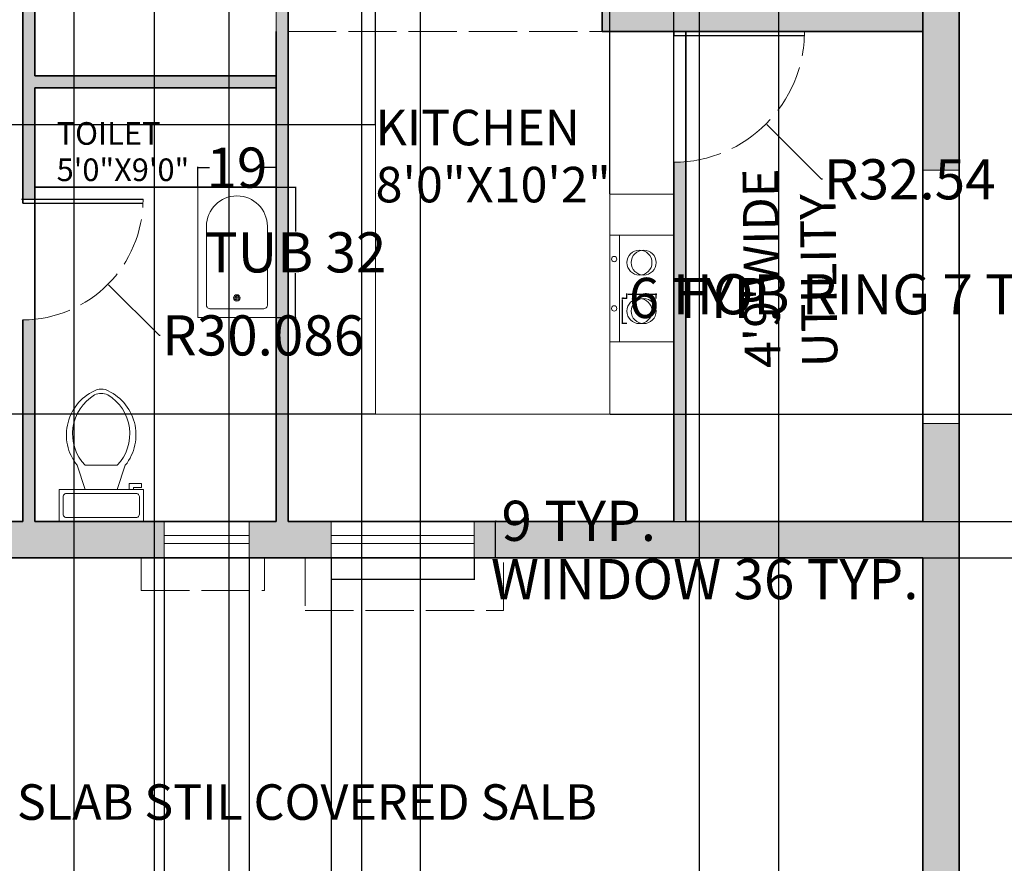
# Model space of a CAD drawing. Units: inches. Extents: x 300 to 1007, y 2 to 1069.
# Tile 9 of 12: x 617 to 862, y 533 to 743. Entities that reach past the tile are written whole.
import ezdxf

# ---------------------------------------------------------------- set-up
doc = ezdxf.new("R2010")
doc.units = ezdxf.units.IN
doc.header["$MEASUREMENT"] = 0
doc.linetypes.add('ACAD_ISO02W100', pattern=[15, 12, -3])
for name, color, linetype, lineweight in [('A-ANNO-DIMS', 2, 'Continuous', 18), ('A-ANNO-TEXT', 7, 'Continuous', 18), ('A-AREA-IDEN', 7, 'Continuous', 18), ('A-CASE', 8, 'Continuous', 18), ('A-DOOR', 3, 'Continuous', 25), ('A-DOOR-SWNG', 3, 'ACAD_ISO02W100', 13), ('A-EQPM', 9, 'Continuous', 18), ('A-FLOR-FIXT', 9, 'Continuous', 18), ('A-FLOR-SLAB', 7, 'Continuous', 35), ('A-GLAZ', 4, 'Continuous', 18), ('A-GLAZ-OVHD', 8, 'ACAD_ISO02W100', 13), ('A-WALL', 7, 'Continuous', 35), ('A-WALL-OVHD', 8, 'ACAD_ISO02W100', 18)]:
    doc.layers.add(name, color=color, linetype=linetype, lineweight=lineweight)
doc.layers.add('A-WALL-PATT', color=9, linetype='Continuous', lineweight=9, true_color=0xc7c8ca)
doc.styles.get("Standard").update_dxf_attribs({"font": 'arial.ttf'})
doc.dimstyles.get("Standard").update_dxf_attribs({"dimtxt": 10, "dimasz": 0.18, "dimexe": 0.18, "dimexo": 0.0625, "dimgap": 0.09, "dimtad": 0, "dimtih": 1, "dimtoh": 1, "dimdec": 0, "dimzin": 0, "dimdsep": 46, "dimlunit": 3, "dimtxsty": 'Standard', "dimcen": 0.09, "dimadec": 0, "dimazin": 0, "dimtfac": 1, "dimtdec": 0, "dimtofl": 0, "dimtmove": 0, "dimatfit": 3, "dimfxl": 1, "dimtolj": 1, "dimtzin": 0, "dimarcsym": 0})

# ---------------------------------------------------------------- blocks, each defined once
blk = doc.blocks.new('Bath Tub - 26 x 60 in.')
for p, q in [((8, -18), (10, -18)), ((9, -17), (9, -19))]:
    blk.add_line(p, q)
blk.add_lwpolyline([(0, -36), (0, 0), (60, 0), (60, -36)], close=True)
for points in [[(6, -4), (42, -4)], [(4, -30), (4, -6)], [(42, -32), (6, -32)]]:
    blk.add_lwpolyline(points)
for radius in [1.5, 1]:
    blk.add_circle((9, -18), radius)
for centre, radius, start, end in [((5.75, -5.75), 1.77, 81.8699, 188.1301), ((42, -18), 14, 270, 90), ((5.75, -30.25), 1.77, 171.8699, 278.1301)]:
    blk.add_arc(centre, radius, start, end)
blk = doc.blocks.new('Toilet - top')
for p, q in [((9.5, -6), (9.5, -2)), ((-10, -8.5), (-8, -8.5)), ((-10, -9.5), (-10, -8.5)), ((-7, -9.5), (-10, -9.5)), ((-8, -8.5), (-8, -8)), ((-7, -8), (-7, -9.5)), ((-4, -8), (-6, -14)), ((4, -8), (6, -14)), ((4, -14), (-4, -14))]:
    blk.add_line(p, q)
blk.add_lwpolyline([(10.5, -8), (10.5, 0), (-10.5, 0), (-10.5, -8)], close=True)
for points in [[(-9.5, -2), (-9.5, -6)], [(8.5, -1), (-8.5, -1)], [(-8.5, -7), (8.5, -7)]]:
    blk.add_lwpolyline(points)
for centre, radius, start, end in [((-8.62, -1.88), 0.884, 81.8699, 188.1301), ((8.62, -1.88), 0.884, 351.8699, 98.1301), ((-8.62, -6.12), 0.884, 171.8699, 278.1301), ((8.62, -6.12), 0.884, 261.8699, 8.1301), ((3.52, -21.58), 12.17, 141.4691, 247.9714), ((4.2, -21.82), 11.33, 136.3677, 238.9468), ((-3.52, -21.58), 12.17, 292.0284, 38.5307), ((-4.2, -21.82), 11.33, 301.053, 43.6321), ((0, -27.88), 4, 245.7318, 294.2682), ((0, -29), 4, 254.8605, 285.1395)]:
    blk.add_arc(centre, radius, start, end)
blk = doc.blocks.new('WIN-35_1-2')
for p, q in [((0, -4.5), (0, 4.5)), ((35.5, 0), (35.5, 4.5)), ((35.5, 4.5), (35.5, -4.5)), ((0, 1), (35.5, 1)), ((0, -1), (35.5, -1))]:
    blk.add_line(p, q)
blk = doc.blocks.new('COOKTOP-RING-6')
for centre in [(0, 0), (1.04, 0)]:
    blk.add_circle(centre, 3.11)
blk = doc.blocks.new('*D41')
at = {"layer": 'A-ANNO-DIMS', "color": 0, "lineweight": -2, "transparency": 16777216}
for p, q in [((680.89, 701.7), (685.87, 701.7)), ((685.69, 701.52), (685.69, 690.67)), ((685.69, 669.43), (685.69, 680.27)), ((680.89, 669.25), (685.87, 669.25))]:
    blk.add_line(p, q, dxfattribs=at)
at = {"layer": 'A-ANNO-DIMS', "color": 0, "transparency": 16777216}
for points in [[(685.66, 701.52), (685.72, 701.52), (685.69, 701.7)], [(685.66, 669.43), (685.72, 669.43), (685.69, 669.25)]]:
    blk.add_solid(points, dxfattribs=at)
at = {"layer": 'Defpoints', "color": 0, "transparency": 16777216}
for p in [(680.83, 701.7), (685.69, 701.7), (680.83, 669.25)]:
    blk.add_point(p, dxfattribs=at)
at = {"layer": 'A-ANNO-DIMS', "color": 0, "transparency": 16777216, "insert": (685.69, 685.47), "char_height": 10, "attachment_point": 5}
blk.add_mtext('\\A1;TUB 32', dxfattribs=at)
blk = doc.blocks.new('*D42')
at = {"layer": 'A-ANNO-DIMS', "color": 0, "lineweight": -2, "transparency": 16777216}
for p, q in [((661.36, 701.76), (661.36, 706.74)), ((661.54, 706.56), (664.3, 706.56)), ((680.65, 706.56), (677.88, 706.56)), ((680.83, 701.76), (680.83, 706.74))]:
    blk.add_line(p, q, dxfattribs=at)
at = {"layer": 'A-ANNO-DIMS', "color": 0, "transparency": 16777216}
for points in [[(661.54, 706.59), (661.54, 706.53), (661.36, 706.56)], [(680.65, 706.59), (680.65, 706.53), (680.83, 706.56)]]:
    blk.add_solid(points, dxfattribs=at)
at = {"layer": 'Defpoints', "color": 0, "transparency": 16777216}
for p in [(661.36, 706.56), (661.36, 701.7), (680.83, 701.7)]:
    blk.add_point(p, dxfattribs=at)
at = {"layer": 'A-ANNO-DIMS', "color": 0, "transparency": 16777216, "insert": (671.09, 706.56), "char_height": 10, "attachment_point": 5}
blk.add_mtext('\\A1;19', dxfattribs=at)
blk = doc.blocks.new('*D61')
at = {"layer": 'A-ANNO-DIMS', "color": 0, "lineweight": -2, "transparency": 16777216}
for p, q in [((694.58, 609.38), (694.58, 603.94)), ((730.11, 609.38), (730.11, 603.94)), ((694.76, 604.12), (729.93, 604.12)), ((730.11, 604.12), (730.29, 604.12))]:
    blk.add_line(p, q, dxfattribs=at)
at = {"layer": 'A-ANNO-DIMS', "color": 0, "transparency": 16777216}
for points in [[(694.76, 604.15), (694.76, 604.09), (694.58, 604.12)], [(729.93, 604.15), (729.93, 604.09), (730.11, 604.12)]]:
    blk.add_solid(points, dxfattribs=at)
at = {"layer": 'Defpoints', "color": 0, "transparency": 16777216}
for p in [(694.58, 609.45), (730.11, 609.45), (730.11, 604.12)]:
    blk.add_point(p, dxfattribs=at)
at = {"layer": 'A-ANNO-DIMS', "color": 0, "transparency": 16777216, "insert": (787.51, 604.12), "char_height": 10, "attachment_point": 5}
blk.add_mtext('\\A1;WINDOW 36 TYP.', dxfattribs=at)
blk = doc.blocks.new('*D62')
at = {"layer": 'A-ANNO-DIMS', "color": 0, "lineweight": -2, "transparency": 16777216}
for p, q in [((730.17, 618.45), (735.62, 618.45)), ((735.44, 618.45), (735.44, 618.63)), ((735.44, 618.63), (735.62, 618.63)), ((735.44, 609.63), (735.44, 618.27)), ((730.17, 609.45), (735.62, 609.45))]:
    blk.add_line(p, q, dxfattribs=at)
at = {"layer": 'A-ANNO-DIMS', "color": 0, "transparency": 16777216}
for points in [[(735.41, 618.27), (735.47, 618.27), (735.44, 618.45)], [(735.41, 609.63), (735.47, 609.63), (735.44, 609.45)]]:
    blk.add_solid(points, dxfattribs=at)
at = {"layer": 'Defpoints', "color": 0, "transparency": 16777216}
for p in [(730.11, 618.45), (735.44, 618.45), (730.11, 609.45)]:
    blk.add_point(p, dxfattribs=at)
at = {"layer": 'A-ANNO-DIMS', "color": 0, "transparency": 16777216, "insert": (756.16, 618.63), "char_height": 10, "attachment_point": 5}
blk.add_mtext('\\A1;9 TYP.', dxfattribs=at)
blk = doc.blocks.new('*D71')
at = {"layer": 'A-ANNO-DIMS', "color": 0, "lineweight": -2, "transparency": 16777216}
for p, q in [((768.17, 674), (768.17, 675.21)), ((768.35, 675.03), (775.25, 675.03)), ((775.43, 674), (775.43, 675.21)), ((775.43, 675.03), (775.61, 675.03))]:
    blk.add_line(p, q, dxfattribs=at)
at = {"layer": 'A-ANNO-DIMS', "color": 0, "transparency": 16777216}
for points in [[(768.35, 675.06), (768.35, 675), (768.17, 675.03)], [(775.25, 675.06), (775.25, 675), (775.43, 675.03)]]:
    blk.add_solid(points, dxfattribs=at)
at = {"layer": 'Defpoints', "color": 0, "transparency": 16777216}
for p in [(768.17, 673.94), (775.43, 675.03), (775.43, 673.94)]:
    blk.add_point(p, dxfattribs=at)
at = {"layer": 'A-ANNO-DIMS', "color": 0, "transparency": 16777216, "insert": (832.37, 675.03), "char_height": 10, "attachment_point": 5}
blk.add_mtext('\\A1;HOB RING 7 TYP.', dxfattribs=at)
blk = doc.blocks.new('*D72')
at = {"layer": 'A-ANNO-DIMS', "color": 0, "lineweight": -2, "transparency": 16777216}
for p, q in [((768.11, 673.94), (766.91, 673.94)), ((767.09, 673.94), (767.09, 674.12)), ((767.09, 674.12), (767.27, 674.12)), ((767.09, 667.9), (767.09, 673.76)), ((768.11, 667.72), (766.91, 667.72))]:
    blk.add_line(p, q, dxfattribs=at)
at = {"layer": 'A-ANNO-DIMS', "color": 0, "transparency": 16777216}
for points in [[(767.06, 673.76), (767.12, 673.76), (767.09, 673.94)], [(767.06, 667.9), (767.12, 667.9), (767.09, 667.72)]]:
    blk.add_solid(points, dxfattribs=at)
at = {"layer": 'Defpoints', "color": 0, "transparency": 16777216}
for p in [(767.09, 673.94), (768.17, 673.94), (768.17, 667.72)]:
    blk.add_point(p, dxfattribs=at)
at = {"layer": 'A-ANNO-DIMS', "color": 0, "transparency": 16777216, "insert": (787.84, 674.12), "char_height": 10, "attachment_point": 5}
blk.add_mtext('\\A1;6 TYP.', dxfattribs=at)
blk = doc.blocks.new('*D77')
at = {"layer": 'A-ANNO-DIMS', "color": 0, "lineweight": -2, "transparency": 16777216}
for p, q in [((841.89, 609.45), (974.48, 609.45)), ((974.3, 609.27), (974.3, 551.11)), ((974.3, 482.56), (974.3, 540.72)), ((850.89, 482.38), (974.48, 482.38))]:
    blk.add_line(p, q, dxfattribs=at)
at = {"layer": 'A-ANNO-DIMS', "color": 0, "transparency": 16777216}
for points in [[(974.27, 609.27), (974.33, 609.27), (974.3, 609.45)], [(974.27, 482.56), (974.33, 482.56), (974.3, 482.38)]]:
    blk.add_solid(points, dxfattribs=at)
at = {"layer": 'Defpoints', "color": 0, "transparency": 16777216}
for p in [(841.83, 609.45), (974.3, 609.45), (850.83, 482.38)]:
    blk.add_point(p, dxfattribs=at)
at = {"layer": 'A-ANNO-DIMS', "color": 0, "transparency": 16777216, "insert": (974.3, 545.92), "char_height": 10, "attachment_point": 5}
blk.add_mtext('\\A1;127.06', dxfattribs=at)
blk = doc.blocks.new('*D78')
at = {"layer": 'A-ANNO-DIMS', "color": 0, "lineweight": -2, "transparency": 16777216}
for p, q in [((850.89, 999.45), (974.48, 999.45)), ((974.3, 999.27), (974.3, 809.65)), ((974.3, 609.63), (974.3, 799.25)), ((841.89, 609.45), (974.48, 609.45))]:
    blk.add_line(p, q, dxfattribs=at)
at = {"layer": 'A-ANNO-DIMS', "color": 0, "transparency": 16777216}
for points in [[(974.27, 999.27), (974.33, 999.27), (974.3, 999.45)], [(974.27, 609.63), (974.33, 609.63), (974.3, 609.45)]]:
    blk.add_solid(points, dxfattribs=at)
at = {"layer": 'Defpoints', "color": 0, "transparency": 16777216}
for p in [(850.83, 999.45), (974.3, 999.45), (841.83, 609.45)]:
    blk.add_point(p, dxfattribs=at)
at = {"layer": 'A-ANNO-DIMS', "color": 0, "transparency": 16777216, "insert": (974.3, 804.45), "char_height": 10, "attachment_point": 5}
blk.add_mtext('\\A1;390', dxfattribs=at)
blk = doc.blocks.new('*D80')
at = {"layer": 'A-ANNO-DIMS', "color": 0, "lineweight": -2, "transparency": 16777216}
for p, q in [((683.83, 717.31), (683.83, 1063.03)), ((684.01, 1062.85), (705.41, 1062.85)), ((705.59, 717.31), (705.59, 1063.03)), ((705.59, 1062.85), (705.77, 1062.85))]:
    blk.add_line(p, q, dxfattribs=at)
at = {"layer": 'A-ANNO-DIMS', "color": 0, "transparency": 16777216}
for points in [[(684.01, 1062.88), (684.01, 1062.82), (683.83, 1062.85)], [(705.41, 1062.88), (705.41, 1062.82), (705.59, 1062.85)]]:
    blk.add_solid(points, dxfattribs=at)
at = {"layer": 'Defpoints', "color": 0, "transparency": 16777216}
for p in [(705.59, 1062.85), (683.83, 717.25), (705.59, 717.25)]:
    blk.add_point(p, dxfattribs=at)
at = {"layer": 'A-ANNO-DIMS', "color": 0, "transparency": 16777216, "insert": (726.71, 1062.85), "char_height": 10, "attachment_point": 5}
blk.add_mtext('\\A1;21.767', dxfattribs=at)
blk = doc.blocks.new('*D81')
at = {"layer": 'A-ANNO-DIMS', "color": 0, "lineweight": -2, "transparency": 16777216}
for p, q in [((705.53, 717.25), (354.19, 717.25)), ((354.37, 717.07), (354.37, 686.41)), ((354.37, 645.35), (354.37, 676.01)), ((705.53, 645.17), (354.19, 645.17))]:
    blk.add_line(p, q, dxfattribs=at)
at = {"layer": 'A-ANNO-DIMS', "color": 0, "transparency": 16777216}
for points in [[(354.34, 717.07), (354.4, 717.07), (354.37, 717.25)], [(354.34, 645.35), (354.4, 645.35), (354.37, 645.17)]]:
    blk.add_solid(points, dxfattribs=at)
at = {"layer": 'Defpoints', "color": 0, "transparency": 16777216}
for p in [(354.37, 717.25), (705.59, 717.25), (705.59, 645.17)]:
    blk.add_point(p, dxfattribs=at)
at = {"layer": 'A-ANNO-DIMS', "color": 0, "transparency": 16777216, "insert": (354.37, 681.21), "char_height": 10, "attachment_point": 5}
blk.add_mtext('\\A1;72.08', dxfattribs=at)
blk = doc.blocks.new('*D82')
at = {"layer": 'A-ANNO-DIMS', "color": 0, "lineweight": -2, "transparency": 16777216}
for p, q in [((763.9, 700.01), (763.9, 1063.03)), ((764.08, 1062.85), (779.65, 1062.85)), ((779.83, 700.01), (779.83, 1063.03)), ((779.83, 1062.85), (780.01, 1062.85))]:
    blk.add_line(p, q, dxfattribs=at)
at = {"layer": 'A-ANNO-DIMS', "color": 0, "transparency": 16777216}
for points in [[(764.08, 1062.88), (764.08, 1062.82), (763.9, 1062.85)], [(779.65, 1062.88), (779.65, 1062.82), (779.83, 1062.85)]]:
    blk.add_solid(points, dxfattribs=at)
at = {"layer": 'Defpoints', "color": 0, "transparency": 16777216}
for p in [(779.83, 1062.85), (763.9, 699.95), (779.83, 699.95)]:
    blk.add_point(p, dxfattribs=at)
at = {"layer": 'A-ANNO-DIMS', "color": 0, "transparency": 16777216, "insert": (800.38, 1062.85), "char_height": 10, "attachment_point": 5}
blk.add_mtext('\\A1;15.927', dxfattribs=at)
blk = doc.blocks.new('*D83')
at = {"layer": 'A-ANNO-DIMS', "color": 0, "lineweight": -2, "transparency": 16777216}
for p, q in [((763.96, 645.17), (974.48, 645.17)), ((974.3, 644.99), (974.3, 637)), ((974.3, 618.63), (974.3, 626.61)), ((779.89, 618.45), (974.48, 618.45))]:
    blk.add_line(p, q, dxfattribs=at)
at = {"layer": 'A-ANNO-DIMS', "color": 0, "transparency": 16777216}
for points in [[(974.27, 644.99), (974.33, 644.99), (974.3, 645.17)], [(974.27, 618.63), (974.33, 618.63), (974.3, 618.45)]]:
    blk.add_solid(points, dxfattribs=at)
at = {"layer": 'Defpoints', "color": 0, "transparency": 16777216}
for p in [(763.9, 645.17), (974.3, 645.17), (779.83, 618.45)]:
    blk.add_point(p, dxfattribs=at)
at = {"layer": 'A-ANNO-DIMS', "color": 0, "transparency": 16777216, "insert": (974.3, 631.81), "char_height": 10, "attachment_point": 5}
blk.add_mtext('\\A1;26.72', dxfattribs=at)
blk = doc.blocks.new('*D86')
at = {"layer": 'A-ANNO-DIMS', "color": 0, "lineweight": -2, "transparency": 16777216}
for p, q in [((805.95, 235.15), (805.95, 1063.03)), ((806.13, 1062.85), (822.02, 1062.85)), ((864.07, 1062.85), (848.18, 1062.85)), ((864.25, 235.15), (864.25, 1063.03))]:
    blk.add_line(p, q, dxfattribs=at)
at = {"layer": 'A-ANNO-DIMS', "color": 0, "transparency": 16777216}
for points in [[(806.13, 1062.88), (806.13, 1062.82), (805.95, 1062.85)], [(864.07, 1062.88), (864.07, 1062.82), (864.25, 1062.85)]]:
    blk.add_solid(points, dxfattribs=at)
at = {"layer": 'Defpoints', "color": 0, "transparency": 16777216}
for p in [(864.25, 1062.85), (805.95, 235.08), (864.25, 235.08)]:
    blk.add_point(p, dxfattribs=at)
at = {"layer": 'A-ANNO-DIMS', "color": 0, "transparency": 16777216, "insert": (835.1, 1062.85), "char_height": 10, "attachment_point": 5}
blk.add_mtext('\\A1;58.3', dxfattribs=at)
blk = doc.blocks.new('*D99')
at = {"layer": 'A-ANNO-DIMS', "color": 0, "lineweight": -2, "transparency": 16777216}
for p, q in [((604.49, 482.45), (604.49, 1063.03)), ((604.67, 1062.85), (619.83, 1062.85)), ((668.97, 1062.85), (653.8, 1062.85)), ((669.15, 482.45), (669.15, 1063.03))]:
    blk.add_line(p, q, dxfattribs=at)
at = {"layer": 'A-ANNO-DIMS', "color": 0, "transparency": 16777216}
for points in [[(604.67, 1062.88), (604.67, 1062.82), (604.49, 1062.85)], [(668.97, 1062.88), (668.97, 1062.82), (669.15, 1062.85)]]:
    blk.add_solid(points, dxfattribs=at)
at = {"layer": 'Defpoints', "color": 0, "transparency": 16777216}
for p in [(669.15, 1062.85), (604.49, 482.38), (669.15, 482.38)]:
    blk.add_point(p, dxfattribs=at)
at = {"layer": 'A-ANNO-DIMS', "color": 0, "transparency": 16777216, "insert": (636.82, 1062.85), "char_height": 10, "attachment_point": 5}
blk.add_mtext('\\A1;64.66', dxfattribs=at)
blk = doc.blocks.new('*D100')
at = {"layer": 'A-ANNO-DIMS', "color": 0, "lineweight": -2, "transparency": 16777216}
for p, q in [((716.78, 482.45), (716.78, 1063.03)), ((716.96, 1062.85), (734.53, 1062.85)), ((786.04, 1062.85), (768.47, 1062.85)), ((786.22, 482.45), (786.22, 1063.03))]:
    blk.add_line(p, q, dxfattribs=at)
at = {"layer": 'A-ANNO-DIMS', "color": 0, "transparency": 16777216}
for points in [[(716.96, 1062.88), (716.96, 1062.82), (716.78, 1062.85)], [(786.04, 1062.88), (786.04, 1062.82), (786.22, 1062.85)]]:
    blk.add_solid(points, dxfattribs=at)
at = {"layer": 'Defpoints', "color": 0, "transparency": 16777216}
for p in [(786.22, 1062.85), (716.78, 482.38), (786.22, 482.38)]:
    blk.add_point(p, dxfattribs=at)
at = {"layer": 'A-ANNO-DIMS', "color": 0, "transparency": 16777216, "insert": (751.5, 1062.85), "char_height": 10, "attachment_point": 5}
blk.add_mtext('\\A1;69.44', dxfattribs=at)
blk = doc.blocks.new('*D102')
at = {"layer": 'A-ANNO-DIMS', "color": 0, "lineweight": -2, "transparency": 16777216}
for p, q in [((600.34, 609.38), (600.34, 8.45)), ((652.99, 609.38), (652.99, 8.45)), ((600.52, 8.63), (609.71, 8.63)), ((652.81, 8.63), (643.62, 8.63))]:
    blk.add_line(p, q, dxfattribs=at)
at = {"layer": 'A-ANNO-DIMS', "color": 0, "transparency": 16777216}
for points in [[(600.52, 8.66), (600.52, 8.6), (600.34, 8.63)], [(652.81, 8.66), (652.81, 8.6), (652.99, 8.63)]]:
    blk.add_solid(points, dxfattribs=at)
at = {"layer": 'Defpoints', "color": 0, "transparency": 16777216}
for p in [(600.34, 609.45), (652.99, 609.45), (652.99, 8.63)]:
    blk.add_point(p, dxfattribs=at)
at = {"layer": 'A-ANNO-DIMS', "color": 0, "transparency": 16777216, "insert": (626.66, 8.63), "char_height": 10, "attachment_point": 5}
blk.add_mtext('\\A1;52.66', dxfattribs=at)
blk = doc.blocks.new('*D103')
at = {"layer": 'A-ANNO-DIMS', "color": 0, "lineweight": -2, "transparency": 16777216}
for p, q in [((652.99, 609.38), (652.99, 8.45)), ((674.16, 609.38), (674.16, 8.45)), ((653.17, 8.63), (673.98, 8.63)), ((674.16, 8.63), (674.34, 8.63))]:
    blk.add_line(p, q, dxfattribs=at)
at = {"layer": 'A-ANNO-DIMS', "color": 0, "transparency": 16777216}
for points in [[(653.17, 8.66), (653.17, 8.6), (652.99, 8.63)], [(673.98, 8.66), (673.98, 8.6), (674.16, 8.63)]]:
    blk.add_solid(points, dxfattribs=at)
at = {"layer": 'Defpoints', "color": 0, "transparency": 16777216}
for p in [(652.99, 609.45), (674.16, 609.45), (674.16, 8.63)]:
    blk.add_point(p, dxfattribs=at)
at = {"layer": 'A-ANNO-DIMS', "color": 0, "transparency": 16777216, "insert": (695.25, 8.63), "char_height": 10, "attachment_point": 5}
blk.add_mtext('\\A1;21.164', dxfattribs=at)
blk = doc.blocks.new('*D104')
at = {"layer": 'A-ANNO-DIMS', "color": 0, "lineweight": -2, "transparency": 16777216}
for p, q in [((674.16, 609.38), (674.16, 8.45)), ((694.58, 609.38), (694.58, 8.45)), ((674.34, 8.63), (694.4, 8.63)), ((694.58, 8.63), (694.76, 8.63))]:
    blk.add_line(p, q, dxfattribs=at)
at = {"layer": 'A-ANNO-DIMS', "color": 0, "transparency": 16777216}
for points in [[(674.34, 8.66), (674.34, 8.6), (674.16, 8.63)], [(694.4, 8.66), (694.4, 8.6), (694.58, 8.63)]]:
    blk.add_solid(points, dxfattribs=at)
at = {"layer": 'Defpoints', "color": 0, "transparency": 16777216}
for p in [(674.16, 609.45), (694.58, 609.45), (694.58, 8.63)]:
    blk.add_point(p, dxfattribs=at)
at = {"layer": 'A-ANNO-DIMS', "color": 0, "transparency": 16777216, "insert": (711.75, 8.63), "char_height": 10, "attachment_point": 5}
blk.add_mtext('\\A1;20.42', dxfattribs=at)
blk = doc.blocks.new('*D106')
at = {"layer": 'A-ANNO-DIMS', "color": 0, "lineweight": -2, "transparency": 16777216}
for p, q in [((582.11, 990.38), (582.11, 8.45)), ((630.49, 990.38), (630.49, 8.45)), ((582.29, 8.63), (589.12, 8.63)), ((630.31, 8.63), (623.47, 8.63))]:
    blk.add_line(p, q, dxfattribs=at)
at = {"layer": 'A-ANNO-DIMS', "color": 0, "transparency": 16777216}
for points in [[(582.29, 8.66), (582.29, 8.6), (582.11, 8.63)], [(630.31, 8.66), (630.31, 8.6), (630.49, 8.63)]]:
    blk.add_solid(points, dxfattribs=at)
at = {"layer": 'Defpoints', "color": 0, "transparency": 16777216}
for p in [(582.11, 990.45), (630.49, 990.45), (630.49, 8.63)]:
    blk.add_point(p, dxfattribs=at)
at = {"layer": 'A-ANNO-DIMS', "color": 0, "transparency": 16777216, "insert": (606.3, 8.63), "char_height": 10, "attachment_point": 5}
blk.add_mtext('\\A1;48.38', dxfattribs=at)
blk = doc.blocks.new('*D107')
at = {"layer": 'A-ANNO-DIMS', "color": 0, "lineweight": -2, "transparency": 16777216}
for p, q in [((630.49, 990.38), (630.49, 8.45)), ((650.47, 990.38), (650.47, 8.45)), ((630.67, 8.63), (650.29, 8.63)), ((650.47, 8.63), (650.65, 8.63))]:
    blk.add_line(p, q, dxfattribs=at)
at = {"layer": 'A-ANNO-DIMS', "color": 0, "transparency": 16777216}
for points in [[(630.67, 8.66), (630.67, 8.6), (630.49, 8.63)], [(650.29, 8.66), (650.29, 8.6), (650.47, 8.63)]]:
    blk.add_solid(points, dxfattribs=at)
at = {"layer": 'Defpoints', "color": 0, "transparency": 16777216}
for p in [(630.49, 990.45), (650.47, 990.45), (650.47, 8.63)]:
    blk.add_point(p, dxfattribs=at)
at = {"layer": 'A-ANNO-DIMS', "color": 0, "transparency": 16777216, "insert": (667.15, 8.63), "char_height": 10, "attachment_point": 5}
blk.add_mtext('\\A1;19.98', dxfattribs=at)
blk = doc.blocks.new('*D108')
at = {"layer": 'A-ANNO-DIMS', "color": 0, "lineweight": -2, "transparency": 16777216}
for p, q in [((650.47, 990.38), (650.47, 8.45)), ((702.09, 990.38), (702.09, 8.45)), ((650.65, 8.63), (659.37, 8.63)), ((701.91, 8.63), (693.19, 8.63))]:
    blk.add_line(p, q, dxfattribs=at)
at = {"layer": 'A-ANNO-DIMS', "color": 0, "transparency": 16777216}
for points in [[(650.65, 8.66), (650.65, 8.6), (650.47, 8.63)], [(701.91, 8.66), (701.91, 8.6), (702.09, 8.63)]]:
    blk.add_solid(points, dxfattribs=at)
at = {"layer": 'Defpoints', "color": 0, "transparency": 16777216}
for p in [(650.47, 990.45), (702.09, 990.45), (702.09, 8.63)]:
    blk.add_point(p, dxfattribs=at)
at = {"layer": 'A-ANNO-DIMS', "color": 0, "transparency": 16777216, "insert": (676.28, 8.63), "char_height": 10, "attachment_point": 5}
blk.add_mtext('\\A1;51.62', dxfattribs=at)
blk = doc.blocks.new('*D115')
at = {"layer": 'A-ANNO-DIMS', "color": 0, "lineweight": -2, "transparency": 16777216}
for p, q in [((779.7, 740.45), (779.88, 740.45)), ((779.79, 740.36), (779.79, 740.54)), ((816.62, 703.66), (802.94, 717.33)), ((816.8, 703.66), (816.62, 703.66))]:
    blk.add_line(p, q, dxfattribs=at)
at = {"layer": 'A-ANNO-DIMS', "color": 0, "transparency": 16777216}
blk.add_solid([(802.96, 717.35), (802.92, 717.3), (802.81, 717.45)], dxfattribs=at)
at = {"layer": 'Defpoints', "color": 0, "transparency": 16777216}
for p in [(779.79, 740.45), (802.81, 717.45)]:
    blk.add_point(p, dxfattribs=at)
at = {"layer": 'A-ANNO-DIMS', "color": 0, "transparency": 16777216, "insert": (838.53, 703.66), "char_height": 10, "attachment_point": 5}
blk.add_mtext('\\A1;R32.54', dxfattribs=at)
blk = doc.blocks.new('*D117')
at = {"layer": 'A-ANNO-DIMS', "color": 0, "lineweight": -2, "transparency": 16777216}
for p, q in [((617.56, 698.73), (617.74, 698.73)), ((617.65, 698.64), (617.65, 698.82)), ((651.79, 664.79), (639.12, 677.39)), ((651.97, 664.79), (651.79, 664.79))]:
    blk.add_line(p, q, dxfattribs=at)
at = {"layer": 'A-ANNO-DIMS', "color": 0, "transparency": 16777216}
blk.add_solid([(639.14, 677.41), (639.09, 677.37), (638.99, 677.52)], dxfattribs=at)
at = {"layer": 'Defpoints', "color": 0, "transparency": 16777216}
for p in [(617.65, 698.73), (638.99, 677.52)]:
    blk.add_point(p, dxfattribs=at)
at = {"layer": 'A-ANNO-DIMS', "color": 0, "transparency": 16777216, "insert": (677.6, 664.79), "char_height": 10, "attachment_point": 5}
blk.add_mtext('\\A1;R30.086', dxfattribs=at)

msp = doc.modelspace()

# ---------------------------------------------------------------- hatches: boundary and pattern name
at = {"layer": 'A-WALL-PATT'}
h = msp.add_hatch(color=256, dxfattribs=at)
h.dxf.hatch_style = 1
h.paths.add_polyline_path([(546.104, 999.4468), (478.8267, 999.4468), (478.8267, 869.2798, -0.06322715), (487.8267, 868.1328), (487.8267, 990.4468), (546.104, 990.4468)])
h.paths.add_polyline_path([(630.4852, 999.4468), (582.106, 999.4468), (582.106, 990.4468), (613.8267, 990.4468), (613.8267, 867.4468), (622.8267, 867.4468), (622.8267, 990.4468), (630.4852, 990.4468)])
h.paths.add_polyline_path([(702.0883, 999.4468), (650.4653, 999.4468), (650.4653, 990.4468), (682.8267, 990.4468), (682.8267, 960.0824, -0.02530575), (685.8267, 960.0478), (685.8267, 990.4468), (702.0883, 990.4468)])
h.paths.add_polyline_path([(850.8267, 999.4468), (737.5888, 999.4468), (737.5888, 990.4468), (841.8267, 990.4468), (841.8267, 950.5685), (850.8267, 950.5685)])
h.paths.add_polyline_path([(685.8267, 930.4465), (682.8267, 930.4465), (682.8267, 888.4468), (682.8267, 867.4468), (685.8267, 867.4468), (697.4169, 867.4468), (697.4169, 870.4468), (685.8267, 870.4468), (685.8267, 888.4468)])
h.paths.add_polyline_path([(682.8267, 931.4465), (654.3436, 931.4465, 0.00843109), (654.3267, 930.4465), (682.8267, 930.4465)])
h.paths.add_polyline_path([(685.8267, 931.4465), (682.8267, 931.4465), (682.8267, 930.4465), (685.8267, 930.4465)])
h.paths.add_polyline_path([(682.8267, 888.4468), (622.8267, 888.4468), (622.8267, 885.4468), (682.8267, 885.4468)])
h.paths.add_polyline_path([(850.8267, 870.4468), (850.8267, 914.7851), (841.8267, 914.7851), (841.8267, 870.4468), (732.7101, 870.4468, -0.02120595), (732.8267, 867.4468), (779.8267, 867.4468), (779.8267, 749.4468), (782.8267, 749.4468), (788.8267, 749.4468), (788.8267, 861.4468), (841.8267, 861.4468), (841.8267, 749.4468), (850.8267, 749.4468)])
h.paths.add_polyline_path([(622.8267, 810.4468), (487.8267, 810.4468), (487.8267, 833.2626), (478.8267, 833.2626), (478.8267, 609.4468), (478.8267, 482.3847), (487.8267, 482.3847), (487.8267, 801.4468), (620.8267, 801.4468), (622.8267, 801.4468)])
h.paths.add_polyline_path([(680.8267, 729.4468), (620.8267, 729.4468), (620.8267, 765.8246, -0.02111352), (617.8267, 766.0562), (617.8267, 698.7303), (620.8267, 698.7303), (620.8267, 726.4468), (680.8267, 726.4468)])
h.paths.add_polyline_path([(620.8267, 668.8122, -0.02498293), (617.8267, 668.6448), (617.8267, 618.4468), (600.3357, 618.4468), (600.3357, 609.4468), (652.9929, 609.4468), (652.9929, 618.4468), (620.8267, 618.4468)])
h.paths.add_polyline_path([(552.3393, 618.4468), (487.8267, 618.4468), (487.8267, 609.4468), (552.3393, 609.4468)], flags=17)
h.paths.add_polyline_path([(694.5763, 618.4468), (683.8267, 618.4468), (683.8267, 726.4468), (683.8267, 749.4468), (680.8267, 749.4468), (680.8267, 740.4468), (680.8267, 726.4468), (680.8267, 618.4468), (674.1573, 618.4468), (674.1573, 609.4468), (680.8267, 609.4468), (694.5763, 609.4468)])
h.paths.add_polyline_path([(850.8267, 642.8902), (841.8267, 642.8902), (841.8267, 618.4468), (782.8267, 618.4468), (782.8267, 708.0513, -0.02308839), (779.8267, 707.9092), (779.8267, 618.4468), (730.1068, 618.4468), (730.1068, 609.4468), (779.8267, 609.4468), (841.8267, 609.4468), (841.8267, 482.3847), (850.8267, 482.3847)])
h.paths.add_polyline_path([(850.8267, 749.4468), (841.8267, 749.4468), (841.8267, 705.9119), (850.8267, 705.9119)])
h.paths.add_polyline_path([(841.8267, 749.4468), (782.8267, 749.4468), (779.8267, 749.4468), (761.9959, 749.4468), (761.9959, 740.4468), (779.8267, 740.4468), (812.3267, 740.4468), (841.8267, 740.4468)])
h.paths.add_polyline_path([(669.1457, 482.3847), (604.489, 482.3847), (604.489, 473.3847), (631.1217, 473.3847), (631.1217, 436.0244, -0.02504709), (634.1217, 436.1748), (634.1217, 436.4367), (634.1217, 473.3847), (669.1457, 473.3847)], flags=17)
h.paths.add_polyline_path([(580.5305, 482.3847), (571.1217, 482.3847), (541.0813, 482.3847), (541.0813, 473.3847), (562.1217, 473.3847), (562.1217, 326.3847), (571.1217, 326.3847), (571.1217, 362.3847), (631.1217, 362.3847), (631.1217, 326.3847), (706.9024, 326.3847, -0.02105388), (706.9999, 329.3847), (634.1217, 329.3847), (634.1217, 365.3847), (634.1217, 406.1748), (631.1217, 406.1748), (631.1217, 365.3847), (571.1217, 365.3847), (571.1217, 473.3847), (580.5305, 473.3847)])
h.paths.add_polyline_path([(493.4756, 482.3847), (420.1217, 482.3847), (420.1217, 445.3134), (429.1217, 445.3134), (429.1217, 473.3847), (493.4756, 473.3847)])
h.paths.add_polyline_path([(786.2236, 482.3847), (716.7793, 482.3847), (716.7793, 473.3847), (766.1217, 473.3847), (766.1217, 329.3847), (742.5583, 329.3847), (742.5583, 326.3847), (766.1217, 326.3847), (766.1217, 316.0647), (769.1217, 316.0647), (769.1217, 326.3847), (769.1217, 473.3847), (786.2236, 473.3847)])
h.paths.add_polyline_path([(910.1217, 482.3847), (822.7166, 482.3847), (822.7166, 473.3847), (901.1217, 473.3847), (901.1217, 402.5393), (910.1217, 402.5393)])
h.paths.add_polyline_path([(910.1217, 366.1034), (901.1217, 366.1034), (901.1217, 329.3847), (814.1217, 329.3847), (814.1217, 312.5176), (817.1217, 312.5176), (817.1217, 326.3847), (901.1217, 326.3847), (901.1217, 293.0319), (910.1217, 293.0319), (910.1217, 326.3847)])
h.paths.add_polyline_path([(910.1217, 268.9355), (901.1217, 268.9355), (901.1217, 254.3847), (817.1217, 254.3847), (817.1217, 290.5411, -0.03396715), (814.1217, 290.3847), (814.1217, 254.3847), (775.1217, 254.3847), (775.1217, 281.5164), (769.1217, 281.5164), (769.1217, 292.1577), (766.1217, 292.1577), (766.1217, 254.3847), (766.1217, 220.1938), (775.5079, 220.1938), (775.5079, 251.3847), (817.1217, 251.3847), (901.1217, 251.3847), (901.1217, 152.3847), (819.0246, 152.3847, -0.02493798), (818.9117, 149.3847), (901.1217, 149.3847), (901.1217, 92.3847), (901.1217, 83.3847), (874.3528, 83.3847), (874.3528, 74.3847), (910.1217, 74.3847), (910.1217, 92.3847), (910.1217, 149.3847)])
h.paths.add_polyline_path([(429.1217, 325.0924), (420.1217, 325.0924), (420.1217, 263.3847), (420.1217, 244.9834), (429.1217, 244.9834), (429.1217, 269.3847), (571.1217, 269.3847), (571.1217, 272.3847), (562.1217, 272.3847), (429.1217, 272.3847)])
h.paths.add_polyline_path([(429.1217, 208.998), (420.1217, 208.998), (420.1217, 74.3847), (496.7704, 74.3847), (496.7704, 83.3847), (429.1217, 83.3847)])
h.paths.add_polyline_path([(598.4322, 83.3847), (571.1217, 83.3847), (571.1217, 122.1171), (562.1217, 122.1171), (562.1217, 83.3847), (544.6031, 83.3847), (544.6031, 74.3847), (598.4322, 74.3847)])
h.paths.add_polyline_path([(797.0822, 83.3847), (769.1217, 83.3847), (769.1217, 149.3847), (788.9123, 149.3847), (788.9123, 152.3847), (769.1217, 152.3847), (769.1217, 178.0167), (766.1217, 178.0167), (766.1217, 152.3847), (735.3598, 152.3847), (735.3598, 143.3847), (766.1217, 143.3847), (766.1217, 83.3847), (634.1217, 83.3847), (634.1217, 143.3847), (659.7326, 143.3847), (659.7326, 152.3847), (634.1217, 152.3847), (634.1217, 194.3847), (571.1217, 194.3847), (571.1217, 233.7289, -0.06379947), (562.1217, 234.7942), (562.1217, 163.4485), (567.7403, 163.4485), (567.7403, 152.3847), (571.1217, 152.3847), (571.1217, 191.3847), (631.1217, 191.3847), (631.1217, 83.3847), (621.979, 83.3847), (621.979, 74.3847), (631.1217, 74.3847), (797.0822, 74.3847)])

# ---------------------------------------------------------------- linework, layer by layer
at = {"layer": 'A-CASE'}
for p, q in [((705.5939, 717.2516), (683.8267, 717.2516)), ((705.5939, 645.167), (705.5939, 717.2516)), ((779.8267, 699.9453), (763.9001, 699.9453)), ((763.9001, 699.9453), (763.9001, 645.167)), ((779.8267, 695.2076), (779.8267, 695.2076)), ((763.9001, 645.167), (683.8267, 645.167))]:
    msp.add_line(p, q, dxfattribs=at)
at = {"layer": 'A-DOOR'}
for p, q in [((779.8267, 740.4468), (779.8267, 740.4468)), ((779.8267, 740.4468), (812.3267, 740.4468)), ((779.8267, 740.4468), (779.8267, 739.4468)), ((779.8267, 739.4468), (779.8267, 740.4468)), ((779.8267, 739.4468), (812.3267, 739.4468)), ((617.8267, 698.7303), (620.8267, 698.7303)), ((617.8267, 698.7303), (647.7386, 698.7303)), ((617.8267, 698.7303), (617.8267, 697.7303)), ((617.8267, 697.7303), (647.7386, 697.7303))]:
    msp.add_line(p, q, dxfattribs=at)
at = {"layer": 'A-DOOR-SWNG'}
for centre, radius, start in [((779.7891, 740.4468), 32.5376, 270.066227), ((617.6526, 698.7303), 30.086, 270.331478)]:
    msp.add_arc(centre, radius, start, 0, dxfattribs=at)
at = {"layer": 'A-EQPM'}
msp.add_line((766.3117, 689.7469), (766.3117, 663.178), dxfattribs=at)
msp.add_lwpolyline([(763.9001, 689.7469), (779.8267, 689.7469), (779.8267, 663.178), (763.9001, 663.178)], close=True, dxfattribs=at)
for centre in [(764.9827, 683.7891), (764.9827, 671.4985)]:
    msp.add_circle(centre, 0.6688, dxfattribs=at)
at = {"layer": 'A-FLOR-SLAB'}
msp.add_line((841.8267, 482.3847), (841.8267, 609.4468), dxfattribs=at)
at = {"layer": 'A-GLAZ'}
for p, q in [((841.8267, 705.9119), (850.8267, 705.9119)), ((841.8267, 642.8902), (850.8267, 642.8902)), ((652.9929, 613.9468), (652.9929, 618.4468)), ((652.9929, 618.4468), (652.9929, 609.4468)), ((674.1573, 618.4468), (674.1573, 609.4468)), ((674.1573, 614.9468), (652.9929, 614.9468)), ((674.1573, 612.9468), (652.9929, 612.9468))]:
    msp.add_line(p, q, dxfattribs=at)
at = {"layer": 'A-GLAZ-OVHD'}
for p, q in [((647.2756, 609.4468), (647.2756, 601.2481)), ((677.9966, 601.2481), (677.9966, 609.4468)), ((688.1022, 609.4468), (688.1022, 596.2858)), ((737.4173, 596.2858), (737.4173, 609.4468)), ((647.2756, 601.2481), (677.9966, 601.2481)), ((688.1022, 596.2858), (737.4173, 596.2858))]:
    msp.add_line(p, q, dxfattribs=at)
at = {"layer": 'A-WALL'}
for p, q in [((617.8267, 697.7303), (617.8267, 766.0562)), ((620.8267, 729.4468), (620.8267, 765.8246)), ((683.8267, 749.4468), (683.8267, 726.4468)), ((761.9959, 749.4468), (761.9959, 740.4468)), ((841.8267, 618.4468), (841.8267, 749.4468)), ((850.8267, 482.3847), (850.8267, 749.4468)), ((680.8267, 740.4468), (680.8267, 726.4468)), ((761.9959, 740.4468), (779.8267, 740.4468)), ((782.8267, 740.4468), (779.8267, 740.4468)), ((782.8267, 618.4468), (782.8267, 740.4468)), ((782.8267, 740.4468), (841.8267, 740.4468)), ((680.8267, 729.4468), (620.8267, 729.4468)), ((620.8267, 618.4468), (620.8267, 726.4468)), ((680.8267, 726.4468), (620.8267, 726.4468)), ((680.8267, 618.4468), (680.8267, 726.4468)), ((683.8267, 618.4468), (683.8267, 726.4468)), ((779.8267, 618.4468), (779.8267, 707.9092)), ((620.8267, 701.6956), (680.8267, 701.6956)), ((617.8267, 618.4468), (617.8267, 668.6448)), ((487.8267, 618.4468), (617.8267, 618.4468)), ((620.8267, 618.4468), (680.8267, 618.4468)), ((683.8267, 618.4468), (779.8267, 618.4468)), ((782.8267, 618.4468), (841.8267, 618.4468)), ((487.8267, 609.4468), (841.8267, 609.4468)), ((620.8267, 609.4468), (680.8267, 609.4468)), ((683.8267, 609.4468), (779.8267, 609.4468)), ((782.8267, 609.4468), (841.8267, 609.4468))]:
    msp.add_line(p, q, dxfattribs=at)
at = {"layer": 'A-WALL-OVHD'}
for p, q in [((680.8267, 749.4468), (680.8267, 740.4468)), ((683.8267, 740.4468), (761.9959, 740.4468))]:
    msp.add_line(p, q, dxfattribs=at)

# ---------------------------------------------------------------- block references
at = {"layer": 'A-EQPM'}
for p in [(771.2833, 682.9152), (771.2833, 670.8302)]:
    msp.add_blockref('COOKTOP-RING-6', p, dxfattribs=at)
at = {"layer": 'A-FLOR-FIXT', "xscale": 0.5408097053283125, "yscale": 0.5408097053283125, "zscale": 0.5408097053283125, "rotation": 90}
msp.add_blockref('Bath Tub - 26 x 60 in.', (661.3576, 669.247), dxfattribs=at)
at = {"layer": 'A-FLOR-FIXT', "rotation": 180}
msp.add_blockref('Toilet - top', (637.3133, 618.4468), dxfattribs=at)
at = {"layer": 'A-GLAZ', "xscale": 1.00084254858565}
msp.add_blockref('WIN-35_1-2', (694.5763, 613.9468), dxfattribs=at)

# ---------------------------------------------------------------- texts
at = {"layer": 'A-ANNO-TEXT'}
msp.add_text('SERVICE SLAB STIL COVERED SALB', height=8.843498, dxfattribs=at).set_placement((566.3949, 544.1919))
at = {"layer": 'A-AREA-IDEN'}
for s, height, p in [('KITCHEN', 8.8435, (705.5939, 712.1152)), ('TOILET', 5.62868, (626.2222, 712.2529)), ('5\'0"X9\'0"', 5.62868, (626.2222, 703.2109)), ('8\'0"X10\'2"', 8.8435, (705.5939, 697.9089))]:
    msp.add_text(s, height=height, dxfattribs=at).set_placement(p)
for s, p in [("4'9'WIDE ", (806.3567, 656.7184)), ('UTILITY', (820.5619, 656.8939))]:
    msp.add_text(s, height=8.8435, rotation=90.707561, dxfattribs=at).set_placement(p)

# ---------------------------------------------------------------- dimensions: what is measured, and where the dimension line sits
at = {"layer": 'A-ANNO-DIMS'}
for base, p1, p2, override, picture, middle in [((669.1457, 1062.8469), (604.489, 482.3847), (669.1457, 482.3847), {"dimdec": 2, "dimlfac": 1, "dimrnd": 0, "dimzin": 0, "dimdsep": 46, "dimlunit": 2}, '*D99', (636.8174, 1062.8469)), ((705.5939, 1062.8469), (683.8267, 717.2516), (705.5939, 717.2516), {"dimdec": 3, "dimlfac": 1, "dimrnd": 0, "dimzin": 0, "dimdsep": 46, "dimlunit": 2}, '*D80', (726.7063, 1062.8469)), ((786.2236, 1062.8469), (716.7793, 482.3847), (786.2236, 482.3847), {"dimdec": 2, "dimlfac": 1, "dimrnd": 0, "dimzin": 0, "dimdsep": 46, "dimlunit": 2}, '*D100', (751.5015, 1062.8469)), ((779.8267, 1062.8469), (763.9001, 699.9453), (779.8267, 699.9453), {"dimdec": 3, "dimlfac": 1, "dimrnd": 0, "dimzin": 0, "dimdsep": 46, "dimlunit": 2}, '*D82', (800.3832, 1062.8469)), ((864.2528, 1062.8469), (805.95, 235.0834), (864.2528, 235.0834), {"dimdec": 1, "dimlfac": 1, "dimrnd": 0, "dimzin": 0, "dimdsep": 46, "dimlunit": 2}, '*D86', (835.1014, 1062.8469)), ((630.4852, 8.6288), (582.106, 990.4468), (630.4852, 990.4468), {"dimdec": 2, "dimlfac": 1, "dimrnd": 0, "dimzin": 0, "dimdsep": 46, "dimlunit": 2}, '*D106', (606.2956, 8.6288)), ((650.4653, 8.6288), (630.4852, 990.4468), (650.4653, 990.4468), {"dimdec": 2, "dimlfac": 1, "dimrnd": 0, "dimzin": 0, "dimdsep": 46, "dimlunit": 2}, '*D107', (667.1473, 8.6288)), ((702.0883, 8.6288), (650.4653, 990.4468), (702.0883, 990.4468), {"dimdec": 2, "dimlfac": 1, "dimrnd": 0, "dimzin": 0, "dimdsep": 46, "dimlunit": 2}, '*D108', (676.2768, 8.6288)), ((652.9929, 8.6288), (600.3357, 609.4468), (652.9929, 609.4468), {"dimdec": 2, "dimlfac": 1, "dimrnd": 0, "dimzin": 0, "dimdsep": 46, "dimlunit": 2}, '*D102', (626.6643, 8.6288)), ((674.1573, 8.6288), (652.9929, 609.4468), (674.1573, 609.4468), {"dimdec": 3, "dimlfac": 1, "dimrnd": 0, "dimzin": 0, "dimdsep": 46, "dimlunit": 2}, '*D103', (695.2493, 8.6288)), ((694.5763, 8.6288), (674.1573, 609.4468), (694.5763, 609.4468), {"dimdec": 2, "dimlfac": 1, "dimrnd": 0, "dimzin": 0, "dimdsep": 46, "dimlunit": 2}, '*D104', (711.7529, 8.6288))]:
    dim = msp.add_linear_dim(base=base, p1=p1, p2=p2, dimstyle='Standard', override=override, dxfattribs=at)
    dim.commit()
    dim.dimension.update_dxf_attribs({"geometry": picture, "text_midpoint": middle})
for base, p1, p2, angle, override, picture, middle in [((974.3023, 999.4468), (841.8267, 609.4468), (850.8267, 999.4468), 90, {"dimdec": 0, "dimlfac": 1, "dimrnd": 0, "dimzin": 0, "dimdsep": 46, "dimlunit": 2}, '*D78', (974.3023, 804.4468)), ((354.3658, 717.2516), (705.5939, 645.167), (705.5939, 717.2516), 90, {"dimdec": 2, "dimlfac": 1, "dimrnd": 0, "dimzin": 0, "dimdsep": 46, "dimlunit": 2}, '*D81', (354.3658, 681.2093)), ((661.3576, 706.5629), (680.8267, 701.6956), (661.3576, 701.6956), 180, {"dimdec": 0, "dimlfac": 1, "dimrnd": 0, "dimzin": 0, "dimdsep": 46, "dimlunit": 2}, '*D42', (671.0921, 706.5629)), ((974.3023, 645.167), (779.8267, 618.4468), (763.9001, 645.167), 90, {"dimdec": 2, "dimlfac": 1, "dimrnd": 0, "dimzin": 0, "dimdsep": 46, "dimlunit": 2}, '*D83', (974.3023, 631.8069)), ((974.3023, 609.4468), (850.8267, 482.3847), (841.8267, 609.4468), 90, {"dimdec": 2, "dimlfac": 1, "dimrnd": 0, "dimzin": 0, "dimdsep": 46, "dimlunit": 2}, '*D77', (974.3023, 545.9158))]:
    dim = msp.add_linear_dim(base=base, p1=p1, p2=p2, angle=angle, dimstyle='Standard', override=override, dxfattribs=at)
    dim.commit()
    dim.dimension.update_dxf_attribs({"geometry": picture, "text_midpoint": middle})
for center, mpoint, override, picture, middle in [((779.7891, 740.4468), (802.8102, 717.4528), {"dimdec": 2, "dimlfac": 1, "dimrnd": 0, "dimzin": 0, "dimdsep": 46, "dimlunit": 2}, '*D115', (838.53, 703.6564)), ((617.6526, 698.7303), (638.9881, 677.5179), {"dimdec": 3, "dimlfac": 1, "dimrnd": 0, "dimzin": 0, "dimdsep": 46, "dimlunit": 2}, '*D117', (677.5982, 664.7905))]:
    dim = msp.add_radius_dim(center=center, mpoint=mpoint, dimstyle='Standard', override=override, dxfattribs=at)
    dim.commit()
    dim.dimension.update_dxf_attribs({"geometry": picture, "text_midpoint": middle, "dimtype": 164})
for base, p1, p2, text, picture, middle in [((775.4308, 675.0284), (768.1736, 673.9399), (775.4308, 673.9399), 'HOB RING <> TYP.', '*D71', (832.3652, 675.0284)), ((730.1068, 604.1172), (694.5763, 609.4468), (730.1068, 609.4468), 'WINDOW <> TYP.', '*D61', (787.5084, 604.1172))]:
    dim = msp.add_linear_dim(base=base, p1=p1, p2=p2, text=text, dimstyle='Standard', override={"dimdec": 0, "dimlfac": 1, "dimrnd": 0, "dimzin": 0, "dimdsep": 46, "dimlunit": 2}, dxfattribs=at)
    dim.commit()
    dim.dimension.update_dxf_attribs({"geometry": picture, "text_midpoint": middle})
for base, p1, p2, text, picture, middle in [((685.694, 701.6956), (680.8267, 669.247), (680.8267, 701.6956), 'TUB <>', '*D41', (685.694, 685.4713)), ((767.085, 673.9399), (768.1736, 667.7205), (768.1736, 673.9399), '<> TYP.', '*D72', (787.8359, 674.1199)), ((735.4363, 618.4468), (730.1068, 609.4468), (730.1068, 618.4468), '<> TYP.', '*D62', (756.16, 618.6268))]:
    dim = msp.add_linear_dim(base=base, p1=p1, p2=p2, angle=90, text=text, dimstyle='Standard', override={"dimdec": 0, "dimlfac": 1, "dimrnd": 0, "dimzin": 0, "dimdsep": 46, "dimlunit": 2}, dxfattribs=at)
    dim.commit()
    dim.dimension.update_dxf_attribs({"geometry": picture, "text_midpoint": middle})

doc.saveas('drawing.dxf')
